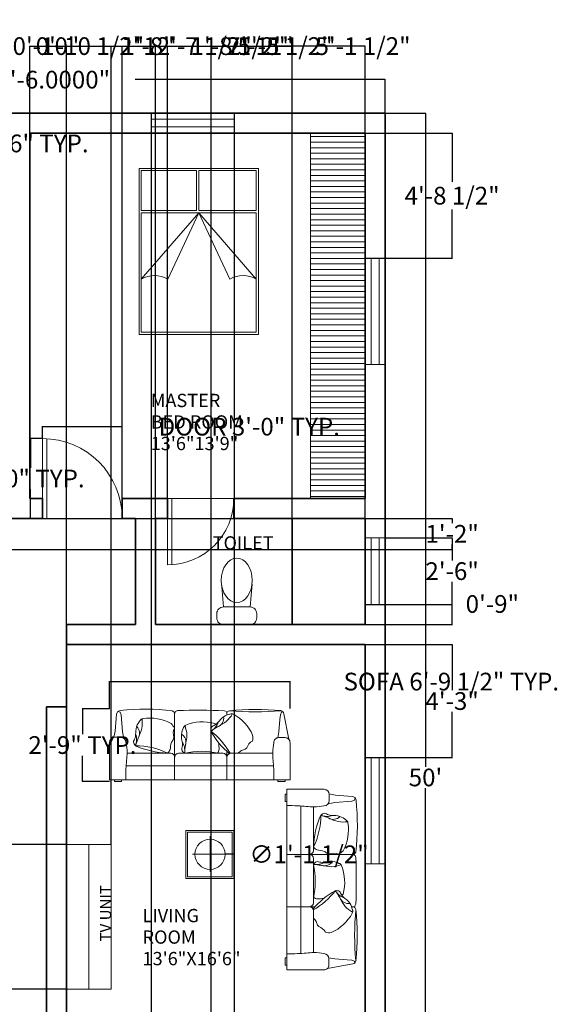
# Model space of a CAD drawing. Units: inches. Extents: x -69 to 405, y -4 to 680.
# Tile 3 of 3: x 162 to 405, y 236 to 680. Entities that reach past the tile are written whole.
import ezdxf

# ---------------------------------------------------------------- set-up
doc = ezdxf.new("R2010")
doc.units = ezdxf.units.IN
doc.header["$MEASUREMENT"] = 0
for name, color, linetype, lineweight in [('A-ANNO-DIMS', 4, 'Continuous', 18), ('A-ANNO-TEXT', 4, 'Continuous', 18), ('A-AREA-IDEN', 4, 'Continuous', 18), ('A-FLOR-CASE', 7, 'Continuous', 18), ('A-FLOR-FIXT', 8, 'Continuous', 18), ('A-WALL', 7, 'Continuous', 35), ('Furniture', 7, 'Continuous', 15)]:
    doc.layers.add(name, color=color, linetype=linetype, lineweight=lineweight)
for name, color, linetype, lineweight, true_color in [('A-DOOR', 2, 'Continuous', 18, 0xf1eb1f), ('A-FLOR-CASE-PATT', 30, 'Continuous', 13, 0xf26722), ('A-GLAZ', 85, 'Continuous', 18, 0x58ba48)]:
    doc.layers.add(name, color=color, linetype=linetype, lineweight=lineweight, true_color=true_color)
doc.styles.get("Standard").update_dxf_attribs({"font": 'italic8.shx'})
doc.dimstyles.get("Standard").update_dxf_attribs({"dimtxt": 8, "dimasz": 0.18, "dimexe": 0.18, "dimexo": 0.0625, "dimgap": 0.09, "dimtad": 0, "dimtih": 1, "dimtoh": 1, "dimdec": 4, "dimzin": 0, "dimdsep": 46, "dimlunit": 3, "dimtxsty": 'Standard', "dimcen": 0.09, "dimadec": 0, "dimazin": 0, "dimtfac": 1, "dimtdec": 4, "dimtofl": 0, "dimtmove": 0, "dimatfit": 3, "dimfxl": 1, "dimtolj": 1, "dimtzin": 0, "dimarcsym": 0})

# ---------------------------------------------------------------- blocks, each defined once
blk = doc.blocks.new('*D4')
at = {"layer": 'A-ANNO-DIMS', "color": 0, "lineweight": -2, "transparency": 16777216}
for p, q in [((21.01, 638.35), (21.01, 653.57)), ((21.19, 653.39), (133.92, 653.39)), ((326.83, 653.39), (214.1, 653.39)), ((327.01, 638.35), (327.01, 653.57))]:
    blk.add_line(p, q, dxfattribs=at)
at = {"layer": 'A-ANNO-DIMS', "color": 0, "transparency": 16777216}
for points in [[(21.19, 653.42), (21.19, 653.36), (21.01, 653.39)], [(326.83, 653.42), (326.83, 653.36), (327.01, 653.39)]]:
    blk.add_solid(points, dxfattribs=at)
at = {"layer": 'Defpoints', "color": 0, "transparency": 16777216}
for p in [(327.01, 653.39), (21.01, 638.28), (327.01, 638.28)]:
    blk.add_point(p, dxfattribs=at)
at = {"layer": 'A-ANNO-DIMS', "color": 0, "transparency": 16777216, "insert": (174.01, 653.39), "char_height": 8, "attachment_point": 5}
blk.add_mtext('\\A1;25\'-6.0000"', dxfattribs=at)
blk = doc.blocks.new('*D5')
at = {"layer": 'A-ANNO-DIMS', "color": 0, "lineweight": -2, "transparency": 16777216}
for p, q in [((327.07, 638.28), (345.4, 638.28)), ((345.22, 638.1), (345.22, 343.14)), ((345.22, 38.46), (345.22, 333.43)), ((327.07, 38.28), (345.4, 38.28))]:
    blk.add_line(p, q, dxfattribs=at)
at = {"layer": 'A-ANNO-DIMS', "color": 0, "transparency": 16777216}
for points in [[(345.19, 638.1), (345.25, 638.1), (345.22, 638.28)], [(345.19, 38.46), (345.25, 38.46), (345.22, 38.28)]]:
    blk.add_solid(points, dxfattribs=at)
at = {"layer": 'Defpoints', "color": 0, "transparency": 16777216}
for p in [(327.01, 638.28), (327.01, 38.28), (345.22, 38.28)]:
    blk.add_point(p, dxfattribs=at)
at = {"layer": 'A-ANNO-DIMS', "color": 0, "transparency": 16777216, "insert": (345.22, 338.28), "char_height": 8, "attachment_point": 5}
blk.add_mtext("\\A1;50'", dxfattribs=at)
blk = doc.blocks.new('SOFA-THREE-SEAT')
for p, q in [((3.69, 30.86, -0.36), (4.84, 31.22, -0.36)), ((29.01, 30.64, -0.36), (28.32, 31.16, -0.36)), ((29.87, 30.79, -0.36), (30.74, 31.2, -0.36)), ((52.77, 30.74, -0.36), (51.91, 31.16, -0.36)), ((53.34, 30.74, -0.36), (54.21, 31.16, -0.36)), ((2.59, 21.95, -0.36), (3.07, 27.61, -0.36)), ((3.07, 27.61, -0.36), (3.23, 29.66, -0.36)), ((3.23, 29.66, -0.36), (3.69, 30.86, -0.36)), ((4.84, 30.5, -0.36), (3.69, 30.86, -0.36)), ((5.3, 29.3, -0.36), (4.84, 30.5, -0.36)), ((5.94, 21.59, -0.36), (5.3, 29.3, -0.36)), ((29.44, 30.02, -0.36), (29.01, 30.64, -0.36)), ((29.43, 0, -0.36), (29.43, 30.03, -0.36)), ((29.44, 30.03, -0.36), (29.87, 30.79, -0.36)), ((53.06, 30.2, -0.36), (52.77, 30.74, -0.36)), ((53.06, 30.2, -0.36), (53.34, 30.74, -0.36)), ((53.06, 30.2, -0.36), (53.06, 29.2, -0.36)), ((76.55, 21.59, -0.36), (77.03, 27.25, -0.36)), ((77.03, 27.25, -0.36), (77.19, 29.3, -0.36)), ((77.19, 29.3, -0.36), (77.65, 30.5, -0.36)), ((77.65, 30.5, -0.36), (78.32, 30.71, -0.36)), ((80.95, 18.3, -0.36), (78.82, 29.77, -0.36)), ((2.01, 18.99, -0.36), (2.59, 21.95, -0.36)), ((2.37, 19.14, -0.36), (5.08, 19.14, -0.36)), ((6.51, 18.64, -0.36), (5.94, 21.59, -0.36)), ((76.04, 18.95, -0.36), (76.55, 21.59, -0.36)), ((79.28, 19, -0.36), (76.57, 19.01, -0.36)), ((0.01, 16.78, -0.36), (0, 0, -0.36)), ((81.57, 0, 13.13), (81.57, 16.63, 13.13)), ((27.66, 11.96, -0.36), (7.88, 11.95, -0.03)), ((51.29, 11.96, -0.36), (31.21, 11.96, -0.36)), ((53.06, 12.74, -0.36), (53.06, 0, -0.36)), ((73.73, 11.96, -0.36), (54.83, 11.96, -0.36)), ((7.53, 6.26, 9.53), (74.14, 6.26, 9.53)), ((81.57, 0, 13.13), (0, 0, -0.36)), ((2.2, 0), (2.2, -0.79)), ((2.2, -0.79), (5.47, -0.79)), ((5.47, -0.79), (5.47, 0, 0.54)), ((76.1, -0.79), (76.1, 0, 0.54)), ((79.37, -0.79), (76.1, -0.79)), ((79.37, 0), (79.37, -0.79))]:
    blk.add_line(p, q)
for centre, radius, start, end in [((16.32, -75.21, -0.36), 107.05, 83.5605, 96.1533), ((40.74, -283.77, -0.36), 315.13, 87.9678, 91.8181), ((65.95, -91.42, -0.36), 123.14, 84.6632, 95.4698), ((65.95, 153.74, -0.36), 123.14, 264.5302, 275.3368), ((77.08, 29.45, -0.36), 1.77, 10.5091, 90), ((15.39, 25.83, 13.13), 1.77, 98.9106, 150.7371), ((18.21, 7.83, 13.13), 19.99, 61.3169, 98.9106), ((47.34, 27.85, 13.13), 4.27, 291.4614, 8.0497), ((55.11, 27.99, 13.13), 1.77, 61.3924, 113.2188), ((46.39, 11.99, 13.13), 19.99, 23.7986, 61.3924), ((9.3, 20.99, 13.13), 4.27, 328.9796, 45.568), ((23.4, 20.62, 13.13), 6.47, 23.6986, 47.1794), ((35.12, 23.03, 13.13), 1.77, 111.9767, 163.8031), ((41.94, 6.13, 13.13), 19.99, 74.3829, 111.9767), ((42.24, 28.19, 13.13), 7.21, 299.4203, 342.7126), ((44.11, 19.77, 13.13), 6.47, 52.7695, 60.2454), ((2.37, 16.78, -0.36), 2.36, 90, 179.9816), ((5.08, 16.78, -0.36), 2.36, 0, 90), ((5.05, 18.15, 13.13), 7.21, 336.9386, 20.2309), ((30.29, 16.94, 13.13), 4.27, 342.0456, 58.634), ((75.47, 38.02, 13.13), 33.78, 208.4934, 231.1155), ((25.19, -4.88, 13.13), 33.78, 29.8342, 52.4564), ((58.3, 18.97, 13.13), 6.47, 346.1804, 9.6612), ((76.56, 16.65, -0.36), 2.36, 89.7859, 179.7859), ((79.31, 16.75, 13.13), 2.25, 357.0581, 90.9206), ((27.22, 50.27, 13.13), 38.25, 246.0331, 268.4688), ((11.67, -18.46, 13.13), 33.78, 64.5272, 89.9746), ((26.79, 13.21, 13.13), 7.21, 350.0046, 33.2969), ((27.66, 10.19, -0.36), 1.77, 0, 90), ((31.21, 10.19, -0.36), 1.77, 90, 180), ((41.52, -20.96, 13.13), 33.78, 76.9593, 103.0407), ((51.29, 10.19, -0.36), 1.77, 0, 90), ((54.83, 10.19, -0.36), 1.77, 90, 180)]:
    blk.add_arc(centre, radius, start, end)
for points, knots in [([(14.37, 27.29, 13.13), (13.69, 26.47, 13.13), (12.22, 24.73, 13.13), (11.75, 21.6, 13.13), (11.87, 18.93, 13.13), (10.39, 16.97, 13.13), (11.27, 15.86, 13.13), (11.69, 15.32, 13.13)], [0, 0, 0, 0, 3.139621, 6.721226, 9.134784, 11.147372, 12.969489, 12.969489, 12.969489, 12.969489]), ([(14.7, 27.34, 13.13), (14.78, 25.95, 13.13), (14.98, 22.92, 13.13), (12.97, 19.11, 13.13), (12.07, 16.46, 13.13), (11.69, 15.32, 13.13)], [0, 0, 0, 0, 4.104513, 8.93575, 12.539242, 12.539242, 12.539242, 12.539242]), ([(55.2, 29.76, 13.13), (54.16, 29.53, 13.13), (51.93, 29.04, 13.13), (49.65, 26.84, 13.13), (48.12, 24.65, 13.13), (45.76, 24, 13.13), (45.77, 22.58, 13.13), (45.78, 21.91, 13.13)], [0, 0, 0, 0, 3.139621, 6.721226, 9.134784, 11.147372, 12.969489, 12.969489, 12.969489, 12.969489]), ([(55.48, 29.6, 13.13), (54.7, 28.44, 13.13), (53.01, 25.93, 13.13), (49.11, 24.13, 13.13), (46.77, 22.57, 13.13), (45.78, 21.91, 13.13)], [0, 0, 0, 0, 4.104513, 8.93575, 12.539242, 12.539242, 12.539242, 12.539242]), ([(29.33, 23.22, 13.13), (29.33, 23.22, 13.13), (28.27, 21.29, 13.13), (29.75, 18.85, 13.13), (27.37, 16.47, 13.13), (27.79, 13.83, 13.13), (26.76, 12.51, 13.13), (26.2, 12.04, 13.13)], [27.786417, 27.786417, 27.786417, 27.786417, 60.334214, 153.42843, 198.910048, 289.238615, 341.466319, 341.466319, 341.466319, 341.466319]), ([(33.81, 24.22, 13.13), (33.33, 23.27, 13.13), (32.29, 21.24, 13.13), (32.54, 18.08, 13.13), (33.26, 15.51, 13.13), (32.26, 13.27, 13.13), (33.37, 12.38, 13.13), (33.9, 11.96, 13.13)], [0, 0, 0, 0, 3.139621, 6.721226, 9.134784, 11.147372, 12.969489, 12.969489, 12.969489, 12.969489]), ([(34.11, 24.34, 13.13), (34.51, 23, 13.13), (35.38, 20.1, 13.13), (34.29, 15.94, 13.13), (34.01, 13.15, 13.13), (33.9, 11.96, 13.13)], [0, 0, 0, 0, 4.104513, 8.93575, 12.539242, 12.539242, 12.539242, 12.539242]), ([(7.47, 16.66, -0.36), (7.71, 15.29, 1.84), (8.23, 12.42, 6.47), (7.36, 5.9, 9.88), (7.38, 1.62, 11.37), (7.39, 0, 11.93)], [0, 0, 0, 0, 7.670782, 16.13452, 21.306634, 21.306634, 21.306634, 21.306634]), ([(49.37, 16.58, 13.13), (49.3, 15.62, 13.13), (49.84, 13.98, 13.13), (49.22, 12.63, 13.13), (48.78, 12.04, 13.13)], [214.332348, 214.332348, 214.332348, 214.332348, 289.238615, 341.466319, 341.466319, 341.466319, 341.466319]), ([(64.59, 17.43, 13.13), (64.59, 17.43, 13.13), (62.57, 16.53, 13.13), (62.25, 13.7, 13.13), (59.48, 13.34, 13.13), (58.61, 12.43, 13.13), (58.17, 11.96, 13.13)], [27.786417, 27.786417, 27.786417, 27.786417, 60.334214, 153.42843, 198.910048, 250.027656, 250.027656, 250.027656, 250.027656]), ([(74.2, 16.66, -0.36), (73.96, 15.29, 1.84), (73.44, 12.42, 6.47), (74.31, 5.9, 9.88), (74.29, 1.62, 11.37), (74.28, 0, 11.93)], [0, 0, 0, 0, 7.670782, 16.13452, 21.306634, 21.306634, 21.306634, 21.306634])]:
    blk.add_open_spline(points, degree=3, knots=knots)
blk = doc.blocks.new('BED-DOUBLE')
for p, q in [((26.03, 55.92), (26.03, 74)), ((27.03, 55.92), (27.03, 74)), ((1, 55.92), (26.03, 55.92)), ((1, 54.92), (53, 54.92)), ((27, 54.92), (1, 25)), ((13, 25), (27, 54.92)), ((27, 54.92), (53, 25)), ((41, 25), (27, 54.92)), ((27.03, 55.92), (53, 55.92))]:
    blk.add_line(p, q)
blk.add_lwpolyline([(0, 75), (54, 75), (54, 0), (0, 0)], close=True)
for points in [[(1, 55.92), (1, 74), (26.03, 74)], [(27.03, 74), (53, 74), (53, 55.92)], [(53, 54.92), (53, 1), (1, 1), (1, 54.92)]]:
    blk.add_lwpolyline(points)
for centre in [(7, 14.51), (47, 14.51)]:
    blk.add_arc(centre, 12.09, 60.2403, 119.7597)
blk = doc.blocks.new('WIN-48IN')
for p, q in [((0, 48), (0, 0)), ((9, 48), (0, 48)), ((2.75, 48), (2.75, 0)), ((6.25, 48), (6.25, 0)), ((9, 0), (9, 48)), ((0, 0), (9, 0))]:
    blk.add_line(p, q)
blk = doc.blocks.new('DOOR-SWING-30IN')
for p, q in [((30, 0), (0, 0)), ((0, 0), (0, -30)), ((2, 0), (2, -29.93))]:
    blk.add_line(p, q)
blk.add_arc((0, 0), 30, 270, 0)
blk = doc.blocks.new('WC-TANK')
for p, q in [((-6, 8), (-6.96, 18.89)), ((6, 8), (6.89, 18.25))]:
    blk.add_line(p, q)
blk.add_lwpolyline([(-6, 0, -0.414214), (-9, 3), (-9, 5, -0.414214), (-6, 8), (6, 8, -0.414214), (9, 5), (9, 3, -0.414214), (6, 0)], format="xyb")
blk.add_ellipse((0, 20), major_axis=(0, 10), ratio=0.7)
blk = doc.blocks.new('DOOR-SWING-36IN')
for p, q in [((0, 0), (0, 36)), ((2, 0), (2, 35.94)), ((36, 0), (0, 0))]:
    blk.add_line(p, q)
blk.add_arc((0, 0), 36, 0, 90)
blk = doc.blocks.new('*D13')
at = {"layer": 'A-ANNO-DIMS', "color": 0, "lineweight": -2, "transparency": 16777216}
for p, q in [((78.15, 613.4), (78.15, 624.76)), ((78.33, 624.58), (131.97, 624.58)), ((132.15, 613.4), (132.15, 624.76)), ((132.15, 624.58), (132.33, 624.58))]:
    blk.add_line(p, q, dxfattribs=at)
at = {"layer": 'A-ANNO-DIMS', "color": 0, "transparency": 16777216}
for points in [[(78.33, 624.61), (78.33, 624.55), (78.15, 624.58)], [(131.97, 624.61), (131.97, 624.55), (132.15, 624.58)]]:
    blk.add_solid(points, dxfattribs=at)
at = {"layer": 'Defpoints', "color": 0, "transparency": 16777216}
for p in [(132.15, 624.58), (78.15, 613.33), (132.15, 613.33)]:
    blk.add_point(p, dxfattribs=at)
at = {"layer": 'A-ANNO-DIMS', "color": 0, "transparency": 16777216, "insert": (168.61, 624.58), "char_height": 8, "attachment_point": 5}
blk.add_mtext('\\A1;4\'-6" TYP.', dxfattribs=at)
blk = doc.blocks.new('*D20')
at = {"layer": 'A-ANNO-DIMS', "color": 0, "lineweight": -2, "transparency": 16777216}
for p, q in [((172.2, 491.35), (172.2, 496.86)), ((172.38, 496.68), (208.02, 496.68)), ((208.2, 491.35), (208.2, 496.86)), ((208.2, 496.68), (208.38, 496.68))]:
    blk.add_line(p, q, dxfattribs=at)
at = {"layer": 'A-ANNO-DIMS', "color": 0, "transparency": 16777216}
for points in [[(172.38, 496.71), (172.38, 496.65), (172.2, 496.68)], [(208.02, 496.71), (208.02, 496.65), (208.2, 496.68)]]:
    blk.add_solid(points, dxfattribs=at)
at = {"layer": 'Defpoints', "color": 0, "transparency": 16777216}
for p in [(208.2, 496.68), (172.2, 491.28), (208.2, 491.28)]:
    blk.add_point(p, dxfattribs=at)
at = {"layer": 'A-ANNO-DIMS', "color": 0, "transparency": 16777216, "insert": (265.61, 496.68), "char_height": 8, "attachment_point": 5}
blk.add_mtext('\\A1;DOOR 3\'-0" TYP.', dxfattribs=at)
blk = doc.blocks.new('*D21')
at = {"layer": 'A-ANNO-DIMS', "color": 0, "lineweight": -2, "transparency": 16777216}
for p, q in [((172.14, 491.28), (166.62, 491.28)), ((166.8, 491.1), (166.8, 478.14)), ((166.8, 455.46), (166.8, 468.43)), ((172.14, 455.28), (166.62, 455.28))]:
    blk.add_line(p, q, dxfattribs=at)
at = {"layer": 'A-ANNO-DIMS', "color": 0, "transparency": 16777216}
for points in [[(166.77, 491.1), (166.83, 491.1), (166.8, 491.28)], [(166.77, 455.46), (166.83, 455.46), (166.8, 455.28)]]:
    blk.add_solid(points, dxfattribs=at)
at = {"layer": 'Defpoints', "color": 0, "transparency": 16777216}
for p in [(166.8, 491.28), (172.2, 491.28), (172.2, 455.28)]:
    blk.add_point(p, dxfattribs=at)
at = {"layer": 'A-ANNO-DIMS', "color": 0, "transparency": 16777216, "insert": (166.8, 473.28), "char_height": 8, "attachment_point": 5}
blk.add_mtext('\\A1;3\'-0" TYP.', dxfattribs=at)
blk = doc.blocks.new('*D22')
at = {"layer": 'A-ANNO-DIMS', "color": 0, "lineweight": -2, "transparency": 16777216}
for p, q in [((202.46, 369.39), (202.46, 381.74)), ((202.64, 381.56), (283.88, 381.56)), ((284.06, 369.39), (284.06, 381.74)), ((284.06, 381.56), (284.24, 381.56))]:
    blk.add_line(p, q, dxfattribs=at)
at = {"layer": 'A-ANNO-DIMS', "color": 0, "transparency": 16777216}
for points in [[(202.64, 381.59), (202.64, 381.53), (202.46, 381.56)], [(283.88, 381.59), (283.88, 381.53), (284.06, 381.56)]]:
    blk.add_solid(points, dxfattribs=at)
at = {"layer": 'Defpoints', "color": 0, "transparency": 16777216}
for p in [(284.06, 381.56), (202.46, 369.32), (284.06, 369.32)]:
    blk.add_point(p, dxfattribs=at)
at = {"layer": 'A-ANNO-DIMS', "color": 0, "transparency": 16777216, "insert": (356.9, 381.56), "char_height": 8, "attachment_point": 5}
blk.add_mtext('\\A1;SOFA 6\'-9 1/2" TYP.', dxfattribs=at)
blk = doc.blocks.new('*D23')
at = {"layer": 'A-ANNO-DIMS', "color": 0, "lineweight": -2, "transparency": 16777216}
for p, q in [((202.4, 369.32), (190.04, 369.32)), ((190.22, 369.14), (190.22, 357.75)), ((190.22, 336.66), (190.22, 348.05)), ((202.4, 336.48), (190.04, 336.48))]:
    blk.add_line(p, q, dxfattribs=at)
at = {"layer": 'A-ANNO-DIMS', "color": 0, "transparency": 16777216}
for points in [[(190.19, 369.14), (190.25, 369.14), (190.22, 369.32)], [(190.19, 336.66), (190.25, 336.66), (190.22, 336.48)]]:
    blk.add_solid(points, dxfattribs=at)
at = {"layer": 'Defpoints', "color": 0, "transparency": 16777216}
for p in [(190.22, 369.32), (202.46, 369.32), (202.46, 336.48)]:
    blk.add_point(p, dxfattribs=at)
at = {"layer": 'A-ANNO-DIMS', "color": 0, "transparency": 16777216, "insert": (190.22, 352.9), "char_height": 8, "attachment_point": 5}
blk.add_mtext('\\A1;2\'-9" TYP.', dxfattribs=at)
blk = doc.blocks.new('*D28')
at = {"layer": 'A-ANNO-DIMS', "color": 0, "lineweight": -2, "transparency": 16777216}
for p, q in [((142.9, 125.35), (142.9, 668.71)), ((143.08, 668.53), (152.72, 668.53)), ((152.9, 125.35), (152.9, 668.71)), ((152.9, 668.53), (153.08, 668.53))]:
    blk.add_line(p, q, dxfattribs=at)
at = {"layer": 'A-ANNO-DIMS', "color": 0, "transparency": 16777216}
for points in [[(143.08, 668.56), (143.08, 668.5), (142.9, 668.53)], [(152.72, 668.56), (152.72, 668.5), (152.9, 668.53)]]:
    blk.add_solid(points, dxfattribs=at)
at = {"layer": 'Defpoints', "color": 0, "transparency": 16777216}
for p in [(152.9, 668.53), (142.9, 125.28), (152.9, 125.28)]:
    blk.add_point(p, dxfattribs=at)
at = {"layer": 'A-ANNO-DIMS', "color": 0, "transparency": 16777216, "insert": (173.75, 668.53), "char_height": 8, "attachment_point": 5}
blk.add_mtext('\\A1;0\'-10"', dxfattribs=at)
blk = doc.blocks.new('*D32')
at = {"layer": 'A-ANNO-DIMS', "color": 0, "lineweight": -2, "transparency": 16777216}
for p, q in [((183.01, 200.35), (183.01, 668.71)), ((183.19, 668.53), (248.2, 668.53)), ((248.38, 200.35), (248.38, 668.71)), ((248.38, 668.53), (248.56, 668.53))]:
    blk.add_line(p, q, dxfattribs=at)
at = {"layer": 'A-ANNO-DIMS', "color": 0, "transparency": 16777216}
for points in [[(183.19, 668.56), (183.19, 668.5), (183.01, 668.53)], [(248.2, 668.56), (248.2, 668.5), (248.38, 668.53)]]:
    blk.add_solid(points, dxfattribs=at)
at = {"layer": 'Defpoints', "color": 0, "transparency": 16777216}
for p in [(248.38, 668.53), (183.01, 200.28), (248.38, 200.28)]:
    blk.add_point(p, dxfattribs=at)
at = {"layer": 'A-ANNO-DIMS', "color": 0, "transparency": 16777216, "insert": (281.8, 668.53), "char_height": 8, "attachment_point": 5}
blk.add_mtext('\\A1;5\'-5 1/2"', dxfattribs=at)
blk = doc.blocks.new('*D37')
at = {"layer": 'A-ANNO-DIMS', "color": 0, "lineweight": -2, "transparency": 16777216}
for p, q in [((223.19, 455.35), (223.19, 668.71)), ((223.37, 668.53), (284.76, 668.53)), ((284.94, 455.35), (284.94, 668.71)), ((284.94, 668.53), (285.12, 668.53))]:
    blk.add_line(p, q, dxfattribs=at)
at = {"layer": 'A-ANNO-DIMS', "color": 0, "transparency": 16777216}
for points in [[(223.37, 668.56), (223.37, 668.5), (223.19, 668.53)], [(284.76, 668.56), (284.76, 668.5), (284.94, 668.53)]]:
    blk.add_solid(points, dxfattribs=at)
at = {"layer": 'Defpoints', "color": 0, "transparency": 16777216}
for p in [(284.94, 668.53), (223.19, 455.28), (284.94, 455.28)]:
    blk.add_point(p, dxfattribs=at)
at = {"layer": 'A-ANNO-DIMS', "color": 0, "transparency": 16777216, "insert": (317.02, 668.53), "char_height": 8, "attachment_point": 5}
blk.add_mtext('\\A1;5\'-1 1/2"', dxfattribs=at)
blk = doc.blocks.new('*D38')
at = {"layer": 'A-ANNO-DIMS', "color": 0, "lineweight": -2, "transparency": 16777216}
for p, q in [((223.19, 407.35), (223.19, 668.71)), ((223.37, 668.53), (251.65, 668.53)), ((317.83, 668.53), (289.55, 668.53)), ((318.01, 407.35), (318.01, 668.71))]:
    blk.add_line(p, q, dxfattribs=at)
at = {"layer": 'A-ANNO-DIMS', "color": 0, "transparency": 16777216}
for points in [[(223.37, 668.56), (223.37, 668.5), (223.19, 668.53)], [(317.83, 668.56), (317.83, 668.5), (318.01, 668.53)]]:
    blk.add_solid(points, dxfattribs=at)
at = {"layer": 'Defpoints', "color": 0, "transparency": 16777216}
for p in [(318.01, 668.53), (223.19, 407.28), (318.01, 407.28)]:
    blk.add_point(p, dxfattribs=at)
at = {"layer": 'A-ANNO-DIMS', "color": 0, "transparency": 16777216, "insert": (270.6, 668.53), "char_height": 8, "attachment_point": 5}
blk.add_mtext('\\A1;7\'-11"', dxfattribs=at)
blk = doc.blocks.new('*D40')
at = {"layer": 'A-ANNO-DIMS', "color": 0, "lineweight": -2, "transparency": 16777216}
for p, q in [((135.01, 407.22), (135.01, 7.85)), ((183.01, 407.22), (183.01, 7.85)), ((135.19, 8.03), (141.01, 8.03)), ((182.83, 8.03), (177, 8.03))]:
    blk.add_line(p, q, dxfattribs=at)
at = {"layer": 'A-ANNO-DIMS', "color": 0, "transparency": 16777216}
for points in [[(135.19, 8.06), (135.19, 8), (135.01, 8.03)], [(182.83, 8.06), (182.83, 8), (183.01, 8.03)]]:
    blk.add_solid(points, dxfattribs=at)
at = {"layer": 'Defpoints', "color": 0, "transparency": 16777216}
for p in [(135.01, 407.28), (183.01, 407.28), (183.01, 8.03)]:
    blk.add_point(p, dxfattribs=at)
at = {"layer": 'A-ANNO-DIMS', "color": 0, "transparency": 16777216, "insert": (159.01, 8.03), "char_height": 8, "attachment_point": 5}
blk.add_mtext('\\A1;4\'-0"', dxfattribs=at)
blk = doc.blocks.new('*D42')
at = {"layer": 'A-ANNO-DIMS', "color": 0, "lineweight": -2, "transparency": 16777216}
for p, q in [((166.51, 629.35), (166.51, 668.71)), ((166.69, 668.53), (206.74, 668.53)), ((317.83, 668.53), (277.78, 668.53)), ((318.01, 629.35), (318.01, 668.71))]:
    blk.add_line(p, q, dxfattribs=at)
at = {"layer": 'A-ANNO-DIMS', "color": 0, "transparency": 16777216}
for points in [[(166.69, 668.56), (166.69, 668.5), (166.51, 668.53)], [(317.83, 668.56), (317.83, 668.5), (318.01, 668.53)]]:
    blk.add_solid(points, dxfattribs=at)
at = {"layer": 'Defpoints', "color": 0, "transparency": 16777216}
for p in [(318.01, 668.53), (166.51, 629.28), (318.01, 629.28)]:
    blk.add_point(p, dxfattribs=at)
at = {"layer": 'A-ANNO-DIMS', "color": 0, "transparency": 16777216, "insert": (242.26, 668.53), "char_height": 8, "attachment_point": 5}
blk.add_mtext('\\A1;12\'-7 1/2"', dxfattribs=at)
blk = doc.blocks.new('*D46')
at = {"layer": 'A-ANNO-DIMS', "color": 0, "lineweight": -2, "transparency": 16777216}
for p, q in [((221.33, 638.22), (221.33, 7.85)), ((258.77, 638.22), (258.77, 7.85)), ((221.51, 8.03), (258.59, 8.03)), ((258.77, 8.03), (258.95, 8.03))]:
    blk.add_line(p, q, dxfattribs=at)
at = {"layer": 'A-ANNO-DIMS', "color": 0, "transparency": 16777216}
for points in [[(221.51, 8.06), (221.51, 8), (221.33, 8.03)], [(258.59, 8.06), (258.59, 8), (258.77, 8.03)]]:
    blk.add_solid(points, dxfattribs=at)
at = {"layer": 'Defpoints', "color": 0, "transparency": 16777216}
for p in [(221.33, 638.28), (258.77, 638.28), (258.77, 8.03)]:
    blk.add_point(p, dxfattribs=at)
at = {"layer": 'A-ANNO-DIMS', "color": 0, "transparency": 16777216, "insert": (290.85, 8.03), "char_height": 8, "attachment_point": 5}
blk.add_mtext('\\A1;3\'-1 1/2"', dxfattribs=at)
blk = doc.blocks.new('*D47')
at = {"layer": 'A-ANNO-DIMS', "color": 0, "lineweight": -2, "transparency": 16777216}
for p, q in [((258.77, 638.22), (258.77, 7.85)), ((327.01, 638.22), (327.01, 7.85)), ((258.95, 8.03), (274.89, 8.03)), ((326.83, 8.03), (310.88, 8.03))]:
    blk.add_line(p, q, dxfattribs=at)
at = {"layer": 'A-ANNO-DIMS', "color": 0, "transparency": 16777216}
for points in [[(258.95, 8.06), (258.95, 8), (258.77, 8.03)], [(326.83, 8.06), (326.83, 8), (327.01, 8.03)]]:
    blk.add_solid(points, dxfattribs=at)
at = {"layer": 'Defpoints', "color": 0, "transparency": 16777216}
for p in [(258.77, 638.28), (327.01, 638.28), (327.01, 8.03)]:
    blk.add_point(p, dxfattribs=at)
at = {"layer": 'A-ANNO-DIMS', "color": 0, "transparency": 16777216, "insert": (292.89, 8.03), "char_height": 8, "attachment_point": 5}
blk.add_mtext('\\A1;5\'-8"', dxfattribs=at)
blk = doc.blocks.new('*D49')
at = {"layer": 'A-ANNO-DIMS', "color": 0, "lineweight": -2, "transparency": 16777216}
for p, q in [((318.07, 629.28), (357.44, 629.28)), ((357.26, 629.1), (357.26, 607.18)), ((357.26, 572.88), (357.26, 594.81)), ((318.07, 572.7), (357.44, 572.7))]:
    blk.add_line(p, q, dxfattribs=at)
at = {"layer": 'A-ANNO-DIMS', "color": 0, "transparency": 16777216}
for points in [[(357.23, 629.1), (357.29, 629.1), (357.26, 629.28)], [(357.23, 572.88), (357.29, 572.88), (357.26, 572.7)]]:
    blk.add_solid(points, dxfattribs=at)
at = {"layer": 'Defpoints', "color": 0, "transparency": 16777216}
for p in [(318.01, 629.28), (318.01, 572.7), (357.26, 572.7)]:
    blk.add_point(p, dxfattribs=at)
at = {"layer": 'A-ANNO-DIMS', "color": 0, "transparency": 16777216, "insert": (357.26, 600.99), "char_height": 8, "attachment_point": 5}
blk.add_mtext('\\A1;4\'-8 1/2"', dxfattribs=at)
blk = doc.blocks.new('*D51')
at = {"layer": 'A-ANNO-DIMS', "color": 0, "lineweight": -2, "transparency": 16777216}
for p, q in [((318.07, 398.28), (357.44, 398.28)), ((357.26, 398.1), (357.26, 377.64)), ((357.26, 347.46), (357.26, 367.93)), ((318.07, 347.28), (357.44, 347.28))]:
    blk.add_line(p, q, dxfattribs=at)
at = {"layer": 'A-ANNO-DIMS', "color": 0, "transparency": 16777216}
for points in [[(357.23, 398.1), (357.29, 398.1), (357.26, 398.28)], [(357.23, 347.46), (357.29, 347.46), (357.26, 347.28)]]:
    blk.add_solid(points, dxfattribs=at)
at = {"layer": 'Defpoints', "color": 0, "transparency": 16777216}
for p in [(318.01, 398.28), (357.26, 398.28), (318.01, 347.28)]:
    blk.add_point(p, dxfattribs=at)
at = {"layer": 'A-ANNO-DIMS', "color": 0, "transparency": 16777216, "insert": (357.26, 372.78), "char_height": 8, "attachment_point": 5}
blk.add_mtext('\\A1;4\'-3"', dxfattribs=at)
blk = doc.blocks.new('*D52')
at = {"layer": 'A-ANNO-DIMS', "color": 0, "lineweight": -2, "transparency": 16777216}
for p, q in [((147.12, 464.35), (147.12, 668.71)), ((147.3, 668.53), (157.33, 668.53)), ((157.51, 464.35), (157.51, 668.71)), ((157.51, 668.53), (157.69, 668.53))]:
    blk.add_line(p, q, dxfattribs=at)
at = {"layer": 'A-ANNO-DIMS', "color": 0, "transparency": 16777216}
for points in [[(147.3, 668.56), (147.3, 668.5), (147.12, 668.53)], [(157.33, 668.56), (157.33, 668.5), (157.51, 668.53)]]:
    blk.add_solid(points, dxfattribs=at)
at = {"layer": 'Defpoints', "color": 0, "transparency": 16777216}
for p in [(157.51, 668.53), (147.12, 464.28), (157.51, 464.28)]:
    blk.add_point(p, dxfattribs=at)
at = {"layer": 'A-ANNO-DIMS', "color": 0, "transparency": 16777216, "insert": (193.59, 668.53), "char_height": 8, "attachment_point": 5}
blk.add_mtext('\\A1;0\'-10 1/2"', dxfattribs=at)
blk = doc.blocks.new('*D53')
at = {"layer": 'A-ANNO-DIMS', "color": 0, "lineweight": -2, "transparency": 16777216}
for p, q in [((208.2, 464.35), (208.2, 668.71)), ((208.38, 668.53), (228.51, 668.53)), ((228.69, 464.35), (228.69, 668.71)), ((228.69, 668.53), (228.87, 668.53))]:
    blk.add_line(p, q, dxfattribs=at)
at = {"layer": 'A-ANNO-DIMS', "color": 0, "transparency": 16777216}
for points in [[(208.38, 668.56), (208.38, 668.5), (208.2, 668.53)], [(228.51, 668.56), (228.51, 668.5), (228.69, 668.53)]]:
    blk.add_solid(points, dxfattribs=at)
at = {"layer": 'Defpoints', "color": 0, "transparency": 16777216}
for p in [(228.69, 668.53), (208.2, 464.28), (228.69, 464.28)]:
    blk.add_point(p, dxfattribs=at)
at = {"layer": 'A-ANNO-DIMS', "color": 0, "transparency": 16777216, "insert": (260.58, 668.53), "char_height": 8, "attachment_point": 5}
blk.add_mtext('\\A1;1\'-8 1/2"', dxfattribs=at)
blk = doc.blocks.new('*D56')
at = {"layer": 'A-ANNO-DIMS', "color": 0, "lineweight": -2, "transparency": 16777216}
for p, q in [((327.07, 446.43), (357.44, 446.43)), ((357.26, 446.25), (357.26, 436.28)), ((357.26, 416.61), (357.26, 426.57)), ((327.07, 416.43), (357.44, 416.43))]:
    blk.add_line(p, q, dxfattribs=at)
at = {"layer": 'A-ANNO-DIMS', "color": 0, "transparency": 16777216}
for points in [[(357.23, 446.25), (357.29, 446.25), (357.26, 446.43)], [(357.23, 416.61), (357.29, 416.61), (357.26, 416.43)]]:
    blk.add_solid(points, dxfattribs=at)
at = {"layer": 'Defpoints', "color": 0, "transparency": 16777216}
for p in [(327.01, 446.43), (357.26, 446.43), (327.01, 416.43)]:
    blk.add_point(p, dxfattribs=at)
at = {"layer": 'A-ANNO-DIMS', "color": 0, "transparency": 16777216, "insert": (357.26, 431.43), "char_height": 8, "attachment_point": 5}
blk.add_mtext('\\A1;2\'-6"', dxfattribs=at)
blk = doc.blocks.new('*D61')
at = {"layer": 'A-ANNO-DIMS', "color": 0, "lineweight": -2, "transparency": 16777216}
for p, q in [((82.63, 455.28), (357.44, 455.28)), ((357.26, 455.1), (357.26, 453.13)), ((82.63, 441.28), (357.44, 441.28)), ((357.26, 441.46), (357.26, 443.43))]:
    blk.add_line(p, q, dxfattribs=at)
at = {"layer": 'A-ANNO-DIMS', "color": 0, "transparency": 16777216}
for points in [[(357.23, 455.1), (357.29, 455.1), (357.26, 455.28)], [(357.23, 441.46), (357.29, 441.46), (357.26, 441.28)]]:
    blk.add_solid(points, dxfattribs=at)
at = {"layer": 'Defpoints', "color": 0, "transparency": 16777216}
for p in [(82.56, 455.28), (82.56, 441.28), (357.26, 441.28)]:
    blk.add_point(p, dxfattribs=at)
at = {"layer": 'A-ANNO-DIMS', "color": 0, "transparency": 16777216, "insert": (357.26, 448.28), "char_height": 8, "attachment_point": 5}
blk.add_mtext('\\A1;1\'-2"', dxfattribs=at)
blk = doc.blocks.new('*D65')
at = {"layer": 'A-ANNO-DIMS', "color": 0, "lineweight": -2, "transparency": 16777216}
for p, q in [((183.01, 307.98), (183.01, 668.71)), ((183.19, 668.53), (203.04, 668.53)), ((203.22, 307.98), (203.22, 668.71)), ((203.22, 668.53), (203.4, 668.53))]:
    blk.add_line(p, q, dxfattribs=at)
at = {"layer": 'A-ANNO-DIMS', "color": 0, "transparency": 16777216}
for points in [[(183.19, 668.56), (183.19, 668.5), (183.01, 668.53)], [(203.04, 668.56), (203.04, 668.5), (203.22, 668.53)]]:
    blk.add_solid(points, dxfattribs=at)
at = {"layer": 'Defpoints', "color": 0, "transparency": 16777216}
for p in [(203.22, 668.53), (183.01, 307.92), (203.22, 307.92)]:
    blk.add_point(p, dxfattribs=at)
at = {"layer": 'A-ANNO-DIMS', "color": 0, "transparency": 16777216, "insert": (219.87, 668.53), "char_height": 8, "attachment_point": 5}
blk.add_mtext('\\A1;1\'-8"', dxfattribs=at)
blk = doc.blocks.new('*D66')
at = {"layer": 'A-ANNO-DIMS', "color": 0, "lineweight": -2, "transparency": 16777216}
for p, q in [((182.95, 307.92), (-9.42, 307.92)), ((-9.24, 307.74), (-9.24, 281.48)), ((-9.24, 242.85), (-9.24, 269.11)), ((182.95, 242.67), (-9.42, 242.67))]:
    blk.add_line(p, q, dxfattribs=at)
at = {"layer": 'A-ANNO-DIMS', "color": 0, "transparency": 16777216}
for points in [[(-9.27, 307.74), (-9.21, 307.74), (-9.24, 307.92)], [(-9.27, 242.85), (-9.21, 242.85), (-9.24, 242.67)]]:
    blk.add_solid(points, dxfattribs=at)
at = {"layer": 'Defpoints', "color": 0, "transparency": 16777216}
for p in [(-9.24, 307.92), (183.01, 307.92), (183.01, 242.67)]:
    blk.add_point(p, dxfattribs=at)
at = {"layer": 'A-ANNO-DIMS', "color": 0, "transparency": 16777216, "insert": (-9.24, 275.29), "char_height": 8, "attachment_point": 5}
blk.add_mtext('\\A1;5\'-5 1/2"', dxfattribs=at)
blk = doc.blocks.new('*D68')
at = {"layer": 'A-ANNO-DIMS', "color": 0, "lineweight": -2, "transparency": 16777216}
for p, q in [((318.07, 416.43), (357.44, 416.43)), ((357.26, 416.43), (357.26, 416.61)), ((357.26, 416.61), (357.44, 416.61)), ((357.26, 407.46), (357.26, 416.25)), ((318.07, 407.28), (357.44, 407.28))]:
    blk.add_line(p, q, dxfattribs=at)
at = {"layer": 'A-ANNO-DIMS', "color": 0, "transparency": 16777216}
for points in [[(357.23, 416.25), (357.29, 416.25), (357.26, 416.43)], [(357.23, 407.46), (357.29, 407.46), (357.26, 407.28)]]:
    blk.add_solid(points, dxfattribs=at)
at = {"layer": 'Defpoints', "color": 0, "transparency": 16777216}
for p in [(318.01, 416.43), (357.26, 416.43), (318.01, 407.28)]:
    blk.add_point(p, dxfattribs=at)
at = {"layer": 'A-ANNO-DIMS', "color": 0, "transparency": 16777216, "insert": (375.43, 416.61), "char_height": 8, "attachment_point": 5}
blk.add_mtext('\\A1;0\'-9"', dxfattribs=at)
blk = doc.blocks.new('*D69')
at = {"layer": 'A-ANNO-DIMS', "color": 0, "lineweight": -2, "transparency": 16777216}
for p, q in [((247.82, 303.56), (248, 303.56)), ((247.91, 303.47), (247.91, 303.65)), ((258.81, 303.56), (254.9, 303.56))]:
    blk.add_line(p, q, dxfattribs=at)
at = {"layer": 'A-ANNO-DIMS', "color": 0, "transparency": 16777216}
blk.add_solid([(254.9, 303.59), (254.9, 303.53), (254.72, 303.56)], dxfattribs=at)
at = {"layer": 'Defpoints', "color": 0, "transparency": 16777216}
for p in [(241.09, 303.56), (254.72, 303.56)]:
    blk.add_point(p, dxfattribs=at)
at = {"layer": 'A-ANNO-DIMS', "color": 0, "transparency": 16777216, "insert": (292.62, 303.56), "char_height": 8, "attachment_point": 5}
blk.add_mtext('\\A1;∅1\'-1 1/2"', dxfattribs=at)

msp = doc.modelspace()

# ---------------------------------------------------------------- hatches: boundary and pattern name
at = {"layer": 'A-FLOR-CASE-PATT'}
h = msp.add_hatch(dxfattribs=at)
h.set_pattern_fill('LINE', color=256, scale=20)
h.set_pattern_definition([(0, (-346.6938, -34.8461), (0, 2.5), [])])
h.paths.add_polyline_path([(56.30318, 629.28441), (30.00851, 629.28441), (30.00851, 464.28441), (56.30318, 464.28441)])
h.paths.add_polyline_path([(318.00851, 629.28441), (293.21188, 629.28441), (293.21188, 464.28441), (318.00851, 464.28441)])

# ---------------------------------------------------------------- linework, layer by layer
at = {"layer": 'A-FLOR-CASE'}
for p, q in [((293.21188, 464.28441), (293.21188, 629.28441)), ((203.21628, 307.92073), (183.00851, 307.92073)), ((193.11239, 242.66874), (193.11239, 307.92073)), ((203.21628, 242.66874), (203.21628, 307.92073)), ((183.00851, 242.66874), (203.21628, 242.66874))]:
    msp.add_line(p, q, dxfattribs=at)
at = {"layer": 'A-GLAZ'}
for p, q in [((221.3312, 638.28441), (221.3312, 629.28441)), ((258.76903, 638.28441), (221.3312, 638.28441)), ((258.76903, 629.28441), (258.76903, 638.28441)), ((221.3312, 635.53441), (258.76903, 635.53441)), ((221.3312, 632.03441), (258.76903, 632.03441)), ((221.3312, 629.28441), (258.76903, 629.28441)), ((318.00851, 416.42557), (318.00851, 446.42557)), ((318.00851, 446.42557), (327.00851, 446.42557)), ((320.75851, 416.42557), (320.75851, 446.42557)), ((324.25851, 416.42557), (324.25851, 446.42557)), ((327.00851, 446.42557), (327.00851, 416.42557)), ((327.00851, 416.42557), (318.00851, 416.42557))]:
    msp.add_line(p, q, dxfattribs=at)
at = {"layer": 'A-WALL'}
for p, q in [((318.00851, 629.28441), (166.50851, 629.28441)), ((166.50851, 464.28441), (166.50851, 629.28441)), ((318.00851, 464.28441), (318.00851, 629.28441)), ((172.20116, 464.28441), (166.50851, 464.28441)), ((172.20116, 455.28441), (172.20116, 464.28441)), ((228.69176, 464.28441), (208.20116, 464.28441)), ((208.20116, 455.28441), (208.20116, 464.28441)), ((228.69176, 455.28441), (228.69176, 464.28441)), ((318.00851, 464.28441), (258.69176, 464.28441)), ((258.69176, 455.28441), (258.69176, 464.28441)), ((172.20116, 455.28441), (147.11856, 455.28441)), ((214.19379, 455.28441), (208.20116, 455.28441)), ((214.19379, 455.28441), (214.19379, 407.28441)), ((223.19379, 455.28441), (223.19379, 407.28441)), ((228.69176, 455.28441), (223.19379, 455.28441)), ((318.00851, 455.28441), (258.69176, 455.28441)), ((284.94096, 455.28441), (284.94096, 407.28441)), ((318.00851, 407.28441), (318.00851, 455.28441)), ((183.00851, 407.28441), (183.00851, 200.28441)), ((214.19379, 407.28441), (183.00851, 407.28441)), ((318.00851, 407.28441), (223.19379, 407.28441)), ((318.00851, 398.28441), (183.00851, 398.28441)), ((318.00851, 200.28441), (318.00851, 398.28441)), ((174.00851, 370.08876), (183.00851, 370.08876)), ((174.00851, 370.08876), (174.00851, 134.28441))]:
    msp.add_line(p, q, dxfattribs=at)
msp.add_lwpolyline([(21.00851, 38.28441), (327.00851, 38.28441), (327.00851, 638.28441), (21.00851, 638.28441)], close=True, dxfattribs=at)
at = {"layer": 'Furniture'}
for p, q in [((236.96125, 314.29031), (258.61475, 314.29031)), ((236.96125, 292.63681), (236.96125, 314.29031)), ((237.74865, 313.50291), (257.82735, 313.50291)), ((237.74865, 293.42421), (237.74865, 313.50291)), ((247.99202, 311.76529), (247.99202, 295.62244)), ((257.82735, 313.50291), (257.82735, 293.42421)), ((258.61475, 314.29031), (258.61475, 292.63681)), ((239.96836, 303.65071), (256.18824, 303.65071)), ((258.61475, 292.63681), (236.96125, 292.63681)), ((257.82735, 293.42421), (237.74865, 293.42421))]:
    msp.add_line(p, q, dxfattribs=at)
msp.add_circle((247.90574, 303.56437), 6.81581, dxfattribs=at)

# ---------------------------------------------------------------- block references
at = {"layer": 'A-DOOR'}
for name, p in [('DOOR-SWING-36IN', (172.20116, 455.28441)), ('DOOR-SWING-30IN', (228.69176, 464.28441))]:
    msp.add_blockref(name, p, dxfattribs=at)
at = {"layer": 'A-FLOR-FIXT'}
msp.add_blockref('WC-TANK', (259.96347, 407.28441), dxfattribs=at)
at = {"layer": 'A-GLAZ'}
for p in [(318.00851, 524.70278), (318.00851, 299.28441)]:
    msp.add_blockref('WIN-48IN', p, dxfattribs=at)
at = {"layer": 'Furniture'}
for name, p in [('BED-DOUBLE', (215.8009, 538.33492)), ('SOFA-THREE-SEAT', (202.46464, 337.26482))]:
    msp.add_blockref(name, p, dxfattribs=at)
at = {"layer": 'Furniture', "rotation": 270}
msp.add_blockref('SOFA-THREE-SEAT', (282.61771, 332.92372), dxfattribs=at)

# ---------------------------------------------------------------- texts
at = {"layer": 'A-ANNO-TEXT'}
msp.add_text('TV UNIT', height=5, rotation=90, dxfattribs=at).set_placement((203.21628, 264.19985))
at = {"layer": 'A-AREA-IDEN'}
for s, p in [('MASTER', (221.08534, 505.51592)), ('BED ROOM', (221.08534, 495.80164)), ('13\'6"13\'9"', (221.08534, 486.08735)), ('TOILET', (249.08936, 441.17775)), ('LIVING', (217.39902, 272.89737)), ('ROOM', (217.39902, 263.18308)), ('13\'6"X16\'6"', (217.39902, 253.4688))]:
    msp.add_text(s, height=6, dxfattribs=at).set_placement(p)

# ---------------------------------------------------------------- dimensions: what is measured, and where the dimension line sits
at = {"layer": 'A-ANNO-DIMS'}
for base, p1, p2, override, picture, middle in [((157.50851, 668.53441), (147.11856, 464.28441), (157.50851, 464.28441), {"dimdec": 1, "dimlfac": 1, "dimrnd": 0, "dimzin": 1, "dimdsep": 46, "dimlunit": 4, "dimfrac": 2}, '*D52', (193.58803, 668.53441)), ((318.00851, 668.53441), (166.50851, 629.28441), (318.00851, 629.28441), {"dimdec": 1, "dimlfac": 1, "dimrnd": 0, "dimzin": 1, "dimdsep": 46, "dimlunit": 4, "dimfrac": 2}, '*D42', (242.25851, 668.53441)), ((248.38397, 668.53441), (183.00851, 200.28441), (248.38397, 200.28441), {"dimdec": 1, "dimlfac": 1, "dimrnd": 0, "dimzin": 1, "dimdsep": 46, "dimlunit": 4, "dimfrac": 2}, '*D32', (281.79683, 668.53441)), ((228.69176, 668.53441), (208.20116, 464.28441), (228.69176, 464.28441), {"dimdec": 1, "dimlfac": 1, "dimrnd": 0, "dimzin": 1, "dimdsep": 46, "dimlunit": 4, "dimfrac": 2}, '*D53', (260.58081, 668.53441)), ((284.94097, 668.53441), (223.19379, 455.28441), (284.94097, 455.28441), {"dimdec": 1, "dimlfac": 1, "dimrnd": 0, "dimzin": 1, "dimdsep": 46, "dimlunit": 4, "dimfrac": 2}, '*D37', (317.02049, 668.53441)), ((152.90475, 668.53441), (142.90475, 125.28441), (152.90475, 125.28441), {"dimdec": 1, "dimlfac": 1, "dimrnd": 0, "dimzin": 1, "dimdsep": 46, "dimlunit": 4, "dimfrac": 2}, '*D28', (173.74618, 668.53441)), ((203.21628, 668.53441), (183.00851, 307.92073), (203.21628, 307.92073), {"dimdec": 1, "dimlfac": 1, "dimrnd": 0, "dimzin": 1, "dimdsep": 46, "dimlunit": 4, "dimfrac": 2}, '*D65', (219.86723, 668.53441)), ((318.00851, 668.53441), (223.19379, 407.28441), (318.00851, 407.28441), {"dimdec": 1, "dimlfac": 1, "dimrnd": 0, "dimzin": 1, "dimdsep": 46, "dimlunit": 4, "dimfrac": 2}, '*D38', (270.60115, 668.53441)), ((327.00851, 653.39083), (21.00851, 638.28441), (327.00851, 638.28441), {"dimclrd": 0, "dimclre": 0, "dimclrt": 0}, '*D4', (174.00851, 653.39083)), ((258.76903, 8.03441), (221.3312, 638.28441), (258.76903, 638.28441), {"dimdec": 1, "dimlfac": 1, "dimrnd": 0, "dimzin": 1, "dimdsep": 46, "dimlunit": 4, "dimfrac": 2}, '*D46', (290.84856, 8.03441)), ((327.00851, 8.03441), (258.76903, 638.28441), (327.00851, 638.28441), {"dimdec": 1, "dimlfac": 1, "dimrnd": 0, "dimzin": 1, "dimdsep": 46, "dimlunit": 4, "dimfrac": 2}, '*D47', (292.88877, 8.03441)), ((183.00851, 8.03441), (135.00851, 407.28441), (183.00851, 407.28441), {"dimdec": 1, "dimlfac": 1, "dimrnd": 0, "dimzin": 1, "dimdsep": 46, "dimlunit": 4, "dimfrac": 2}, '*D40', (159.00851, 8.03441))]:
    dim = msp.add_linear_dim(base=base, p1=p1, p2=p2, dimstyle='Standard', override=override, dxfattribs=at)
    dim.commit()
    dim.dimension.update_dxf_attribs({"geometry": picture, "text_midpoint": middle})
for base, p1, p2, text, picture, middle in [((132.1517, 624.58492), (78.1517, 613.33492), (132.1517, 613.33492), '<> TYP.', '*D13', (168.61218, 624.58492)), ((208.20116, 496.68441), (172.20116, 491.28441), (208.20116, 491.28441), 'DOOR <> TYP.', '*D20', (265.61401, 496.68441)), ((284.06283, 381.56334), (202.46464, 369.32361), (284.06283, 369.32361), 'SOFA <> TYP.', '*D22', (356.90426, 381.56334))]:
    dim = msp.add_linear_dim(base=base, p1=p1, p2=p2, text=text, dimstyle='Standard', override={"dimdec": 1, "dimlfac": 1, "dimrnd": 0, "dimzin": 1, "dimdsep": 46, "dimlunit": 4, "dimfrac": 2}, dxfattribs=at)
    dim.commit()
    dim.dimension.update_dxf_attribs({"geometry": picture, "text_midpoint": middle})
for base, p1, p2, override, picture, middle in [((345.22225, 38.28441), (327.00851, 638.28441), (327.00851, 38.28441), {"dimclrd": 0, "dimclre": 0, "dimclrt": 0}, '*D5', (345.22225, 338.28441)), ((357.25851, 572.70278), (318.00851, 629.28441), (318.00851, 572.70278), {"dimdec": 1, "dimlfac": 1, "dimrnd": 0, "dimzin": 1, "dimdsep": 46, "dimlunit": 4, "dimfrac": 2}, '*D49', (357.25851, 600.9936)), ((357.25851, 441.28014), (82.56355, 455.28441), (82.56355, 441.28014), {"dimdec": 1, "dimlfac": 1, "dimrnd": 0, "dimzin": 1, "dimdsep": 46, "dimlunit": 4, "dimfrac": 2}, '*D61', (357.25851, 448.28227)), ((357.25851, 446.42557), (327.00851, 416.42557), (327.00851, 446.42557), {"dimdec": 1, "dimlfac": 1, "dimrnd": 0, "dimzin": 1, "dimdsep": 46, "dimlunit": 4, "dimfrac": 2}, '*D56', (357.25851, 431.42557)), ((357.25851, 416.42557), (318.00851, 407.28441), (318.00851, 416.42557), {"dimdec": 1, "dimlfac": 1, "dimrnd": 0, "dimzin": 1, "dimdsep": 46, "dimlunit": 4, "dimfrac": 2}, '*D68', (375.43327, 416.60557)), ((357.25851, 398.28441), (318.00851, 347.28441), (318.00851, 398.28441), {"dimdec": 1, "dimlfac": 1, "dimrnd": 0, "dimzin": 1, "dimdsep": 46, "dimlunit": 4, "dimfrac": 2}, '*D51', (357.25851, 372.78441)), ((-9.24149, 307.92073), (183.00851, 242.66874), (183.00851, 307.92073), {"dimdec": 1, "dimlfac": 1, "dimrnd": 0, "dimzin": 1, "dimdsep": 46, "dimlunit": 4, "dimfrac": 2}, '*D66', (-9.24149, 275.29473))]:
    dim = msp.add_linear_dim(base=base, p1=p1, p2=p2, angle=90, dimstyle='Standard', override=override, dxfattribs=at)
    dim.commit()
    dim.dimension.update_dxf_attribs({"geometry": picture, "text_midpoint": middle})
for base, p1, p2, picture, middle in [((166.80116, 491.28441), (172.20116, 455.28441), (172.20116, 491.28441), '*D21', (166.80116, 473.28441)), ((190.22491, 369.32361), (202.46464, 336.47854), (202.46464, 369.32361), '*D23', (190.22491, 352.90107))]:
    dim = msp.add_linear_dim(base=base, p1=p1, p2=p2, angle=90, text='<> TYP.', dimstyle='Standard', override={"dimdec": 1, "dimlfac": 1, "dimrnd": 0, "dimzin": 1, "dimdsep": 46, "dimlunit": 4, "dimfrac": 2}, dxfattribs=at)
    dim.commit()
    dim.dimension.update_dxf_attribs({"geometry": picture, "text_midpoint": middle})
dim = msp.add_diameter_dim_2p(p1=(241.08994, 303.56474), p2=(254.72155, 303.564), dimstyle='Standard', override={"dimdec": 1, "dimlfac": 1, "dimrnd": 0, "dimzin": 1, "dimdsep": 46, "dimlunit": 4, "dimfrac": 2}, dxfattribs=at)
dim.commit()
dim.dimension.update_dxf_attribs({"geometry": '*D69', "text_midpoint": (258.81104, 303.56378), "dimtype": 163})

doc.saveas('drawing.dxf')
